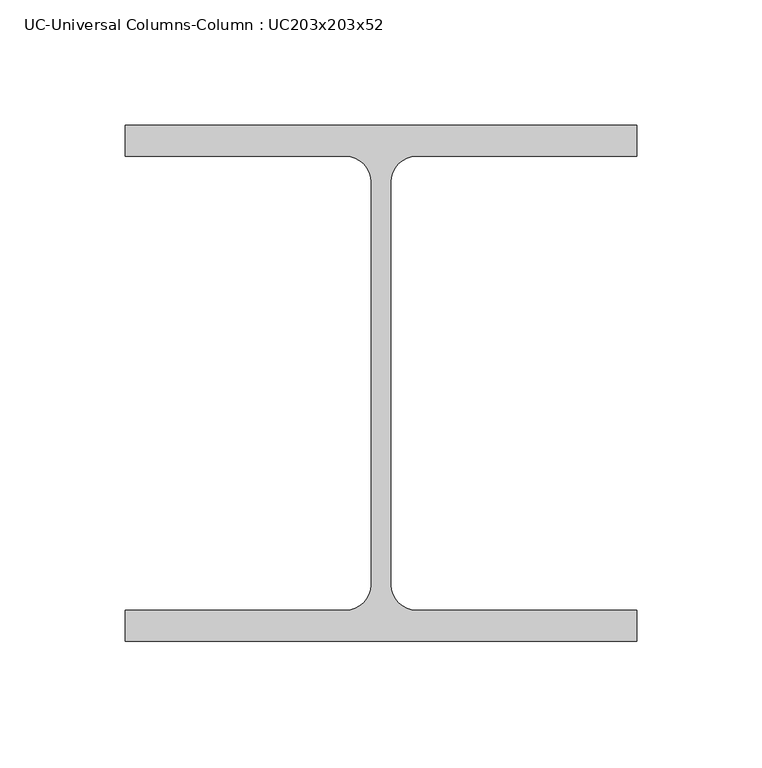
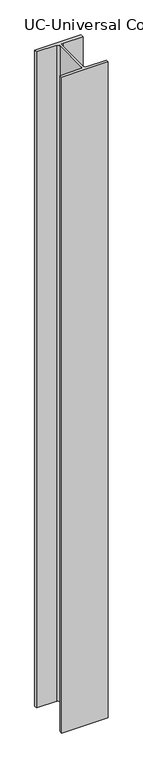
"""IFC4 building model written with IfcOpenShell, lengths in millimetres: column geometry, UC-Universal Columns-Column : UC203x203x52."""

from ifc_helpers import new_model, si_unit, point, frame, frame_2d, origin, place, context, project, spatial, polyline, circle_curve, trimmed, segment, composite_curve, outline, extrude, source, transform, mapped, element, save


def uc_universal_columns_column_uc203x203x52_fec190f4(model_context):
    return source(origin(), model_context, "Body", "SweptSolid", [
        extrude(outline(composite_curve([segment(polyline([(102.15, 103.1), (102.15, 90.6), (14.15, 90.6)]), True, "CONTINUOUS"), segment(trimmed(circle_curve(frame_2d((14.15, 80.4)), 10.2), [point((14.15, 90.6))], [point((3.95, 80.4))], True, "CARTESIAN"), True, "CONTINUOUS"), segment(polyline([(3.95, 80.4), (3.95, -80.4)]), True, "CONTINUOUS"), segment(trimmed(circle_curve(frame_2d((14.15, -80.4)), 10.2), [point((3.95, -80.4))], [point((14.15, -90.6))], True, "CARTESIAN"), True, "CONTINUOUS"), segment(polyline([(14.15, -90.6), (102.15, -90.6), (102.15, -103.1), (-102.15, -103.1), (-102.15, -90.6), (-14.15, -90.6)]), True, "CONTINUOUS"), segment(trimmed(circle_curve(frame_2d((-14.15, -80.4)), 10.2), [point((-14.15, -90.6))], [point((-3.95, -80.4))], True, "CARTESIAN"), True, "CONTINUOUS"), segment(polyline([(-3.95, -80.4), (-3.95, 80.4)]), True, "CONTINUOUS"), segment(trimmed(circle_curve(frame_2d((-14.15, 80.4)), 10.2), [point((-3.95, 80.4))], [point((-14.15, 90.6))], True, "CARTESIAN"), True, "CONTINUOUS"), segment(polyline([(-14.15, 90.6), (-102.15, 90.6), (-102.15, 103.1), (102.15, 103.1)]), True, "CONTINUOUS")], self_intersect=False)), frame((0.0, 0.0, 3048.0), z_axis=(0.0, 0.0, 1.0), x_axis=(1.0, 0.0, 0.0)), (0.0, 0.0, 1.0), 3048.0),
    ])


if __name__ == "__main__":
    model = new_model("IFC4")
    model_context = context("Model", 3, world=origin())
    ifc_project = project(units=[si_unit("LENGTHUNIT", "METRE", prefix="MILLI")], contexts=[model_context])
    site = spatial("IfcSite", under=ifc_project)
    building = spatial("IfcBuilding", under=site)
    placement = place(None, origin())
    uc_universal_columns_column_uc203x203x52_shape = uc_universal_columns_column_uc203x203x52_fec190f4(model_context)
    element("IfcColumn", 1, ObjectType="UC-Universal Columns-Column : UC203x203x52", at=placement, inside=building, context=model_context, shape_type="MappedRepresentation", body=[
        mapped(uc_universal_columns_column_uc203x203x52_shape, transform((0.0, 0.0, 0.0), x_axis=(1.0, 0.0, 0.0), y_axis=(0.0, 1.0, 0.0), z_axis=(0.0, 0.0, 1.0))),
    ])
    save(model, "model.ifc")

# Revit data of these elements
# Type "UC-Universal Columns-Column : UC203x203x52"
#   Section Name Key = "UC203x203x52"
#   Width = 20.43 cm
#   Web Thickness = 0.79 cm
#   Web Fillet = 1.02 cm
#   Warping Constant = 167000.0 cm⁶
#   Torsional Moment of Inertia = 31.80 cm⁴
#   Section Area = 66.0 cm²
#   Plastic Modulus weak axis = 264.0 cm³
#   Plastic Modulus strong axis = 567.0 cm³
#   Nominal Weight = 51.9998 kgf/m
#   Moment of Inertia weak axis = 1778.00 cm⁴
#   Moment of Inertia strong axis = 5259.00 cm⁴
#   Height = 20.62 cm
#   Flange Thickness = 1.25 cm
#   Elastic Modulus weak axis = 174.0 cm³
#   Elastic Modulus strong axis = 510.0 cm³
#   Centroid Vertical = 10.31 cm
#   Centroid Horizontal = 10.215 cm
#   Bolt Spacing = 14.0 cm
#   Structural Material [instance default] = Metal - Steel 43-275
#   Type Comments = ""
#   Assembly Code = ""
# Element 1 (IfcColumn, "UC-Universal Columns-Column : UC203x203x52")
#   Materials on its faces: "Metal - Steel 43-275"
# Materials
#   "Metal - Steel 43-275": class "Metal", colour RGB 247 247 247, transparency 0, Cost = 0
